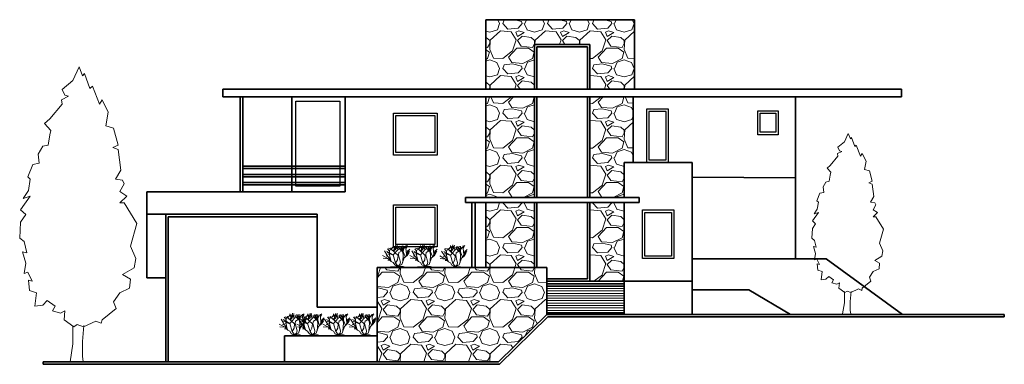
# Model space of a CAD drawing. Units: inches. Extents: x -92 to 721, y 126 to 411.
import ezdxf

# ---------------------------------------------------------------- set-up
doc = ezdxf.new("R2010")
doc.units = ezdxf.units.IN
doc.header["$MEASUREMENT"] = 0
for name, color, linetype, lineweight in [('A-ELEV', 7, 'Continuous', 35), ('A-FLOR-STRS', 3, 'Continuous', 18), ('A-GLAZ', 4, 'Continuous', 25), ('A-WALL-PATT', 8, 'Continuous', 13), ('L-PLNT', 3, 'Continuous', 13)]:
    doc.layers.add(name, color=color, linetype=linetype, lineweight=lineweight)

# ---------------------------------------------------------------- blocks, each defined once
blk = doc.blocks.new('*U2')
blk.add_lwpolyline([(-2.754, 191.699), (-6.78, 182.851), (-13.682, 176.953), (-11.956, 173.266), (-9.656, 172.529), (-14.257, 170.317), (-13.682, 167.368), (-21.733, 157.783), (-25.184, 154.834), (-21.158, 150.41), (-21.733, 147.461), (-22.884, 140.825), (-26.334, 140.087), (-29.21, 134.926), (-28.635, 129.028), (-32.661, 128.291), (-36.111, 120.18), (-34.386, 118.706), (-35.536, 111.333), (-38.987, 106.171), (-34.386, 107.646), (-40.712, 98.798), (-37.261, 95.849), (-40.712, 90.688), (-41.287, 80.366), (-38.412, 78.154), (-36.686, 70.781), (-39.562, 71.518), (-37.261, 64.145), (-38.412, 57.509), (-36.111, 58.247), (-33.236, 52.348), (-35.536, 53.086), (-34.961, 46.45), (-30.36, 44.975), (-31.51, 36.128), (-26.334, 36.865), (-23.459, 39.814), (-18.283, 36.128), (-20.008, 33.178), (-14.832, 31.704), (-11.956, 33.178), (-12.531, 27.28), (-6.205, 22.856), (-3.905, 24.331), (0.121, 22.856), (8.173, 26.543), (11.624, 25.068), (12.199, 27.28), (21.4, 34.653), (19.675, 39.077), (23.701, 44.975), (30.027, 47.924), (30.602, 53.823), (25.426, 56.772), (32.903, 61.196), (34.053, 67.094), (30.602, 75.205), (34.628, 89.951), (26.576, 103.222), (23.701, 103.222), (28.302, 107.646), (23.701, 110.595), (26.576, 115.756), (25.426, 117.968), (20.825, 118.706), (24.276, 124.604), (22.551, 137.876), (19.1, 139.35), (22.551, 140.825), (19.675, 151.884), (14.499, 153.359), (16.224, 162.207), (12.199, 170.317), (10.473, 167.368), (5.872, 179.165), (4.147, 177.69), (0.696, 187.275), (-0.454, 185.8)], close=True)
for points in [[(-6.813, 23.669), (-6.813, 11.669), (-8.627, 0)], [(0.387, 23.669), (-0.576, 13.271), (-0.576, 3.686), (0, 0)]]:
    blk.add_lwpolyline(points)
blk = doc.blocks.new('*U3')
for p, q in [((-14.88, 18.24), (-12.96, 20.64)), ((-12.471, 19.775), (-12.898, 22.044)), ((-11.677, 19.071), (-12.471, 19.775)), ((-11.28, 19.619), (-12.104, 21.184)), ((-11.921, 18.836), (-10.64, 20.401)), ((-11.433, 18.289), (-10.457, 22.749)), ((-10.579, 18.054), (-9.846, 19.697)), ((-8.16, 17.76), (-10.56, 21.6)), ((-9.48, 19.775), (-8.992, 22.592)), ((-7.2, 19.68), (-8.64, 20.16)), ((-7.2, 19.68), (-6.24, 21.12)), ((-5.086, 17.741), (-5.513, 21.34)), ((-5.28, 19.2), (-3.84, 21.6)), ((-3.84, 16.8), (-0.96, 20.64)), ((-3.377, 18.602), (-2.888, 21.575)), ((-2.88, 15.84), (-2.4, 20.16)), ((-0.508, 21.888), (-0.081, 20.558)), ((-0.203, 19.149), (0.102, 21.34)), ((-0.142, 19.384), (0.59, 20.401)), ((-0.02, 20.01), (0.896, 21.105)), ((0.041, 20.714), (1.384, 22.044)), ((0.102, 21.34), (0.835, 21.888)), ((-17.76, 8.64), (-23.663, 11.961)), ((-18.24, 11.04), (-21.755, 16.655)), ((-18.24, 11.04), (-20.16, 11.52)), ((-12.96, 12.48), (-19.68, 16.32)), ((-13.92, 12.48), (-19.2, 14.88)), ((-16.8, 16.32), (-18.72, 18.72)), ((-15.84, 8.16), (-18.24, 11.04)), ((-14.88, 18.24), (-17.76, 19.2)), ((-16.8, 12.48), (-17.76, 12.96)), ((-16.8, 16.32), (-15.36, 19.68)), ((-16.8, 12.48), (-16.8, 16.32)), ((-15.84, 8.16), (-16.8, 12.48)), ((-8.16, 12), (-14.88, 18.24)), ((-12.96, 12.48), (-13.92, 12.48)), ((-13.325, 16.724), (-11.433, 18.289)), ((-12.96, 12.48), (-8.16, 17.76)), ((-10.56, 4.32), (-12.96, 12.48)), ((-12.043, 15.628), (-11.921, 18.836)), ((-11.982, 16.802), (-10.579, 18.054)), ((-8.64, 7.68), (-8.16, 12)), ((-8.16, 17.76), (-5.28, 19.2)), ((-7.68, 12.48), (-7.2, 14.88)), ((-6.72, 8.64), (-7.68, 12.48)), ((-4.8, 16.32), (-7.2, 19.68)), ((-7.2, 14.88), (-3.84, 16.8)), ((-3.377, 15.315), (-5.086, 17.819)), ((-2.88, 12.96), (-4.32, 19.68)), ((-2.766, 16.802), (-3.377, 18.602)), ((-3.36, 5.28), (-2.88, 12.96)), ((-0.96, 10.56), (-2.88, 15.84)), ((-1.92, 9.6), (0.96, 12)), ((-0.48, 10.8), (0.346, 13.203)), ((0.346, 13.203), (-0.203, 19.149)), ((0.346, 13.203), (1.323, 16.254)), ((0.96, 12), (1.44, 15.36)), ((0.96, 12), (2.88, 14.88)), ((1.323, 16.254), (3.642, 18.289)), ((1.44, 15.36), (2.88, 17.28)), ((1.92, 13.44), (2.4, 15.36)), ((2.4, 15.36), (3.36, 16.32)), ((-17.76, 8.64), (-23.128, 9.222)), ((-16.32, 7.2), (-18.24, 7.2)), ((-14.88, 5.76), (-17.76, 8.64)), ((-15.84, 0.48), (-17.76, 0)), ((-14.88, 5.76), (-15.84, 8.16)), ((-13.44, 0.48), (-15.84, 0.48)), ((-12.96, 4.8), (-14.88, 5.76)), ((-9.6, 0.96), (-13.44, 0.48)), ((-11.52, 2.4), (-12.96, 4.8)), ((-9.6, 0.96), (-12.96, 0)), ((-8.64, 0.96), (-11.52, 2.4)), ((-10.56, 4.32), (-8.64, 7.68)), ((-8.64, 1.92), (-10.56, 4.32)), ((-9.6, 0.96), (-7.68, 0.96)), ((-8.64, 0.96), (-4.32, 2.88)), ((-8.64, 0.96), (-6.24, 2.88)), ((-8.64, 0.96), (-8.64, 1.92)), ((-8.64, 0.96), (-2.88, 0.96)), ((-7.68, 0.96), (-6.24, 0.48)), ((-5.76, 5.28), (-6.72, 8.64)), ((-6.24, 2.88), (-5.76, 5.28)), ((-6.24, 0.48), (-3.36, 0)), ((-4.32, 2.88), (-1.92, 9.6)), ((-2.88, 0.96), (0, 0))]:
    blk.add_line(p, q)

msp = doc.modelspace()

# ---------------------------------------------------------------- hatches: boundary and pattern name
at = {"layer": 'A-WALL-PATT'}
h = msp.add_hatch(dxfattribs=at)
h.set_pattern_fill('GRAVEL', color=256, scale=37)
h.paths.add_polyline_path([(343.25, 205.86), (203.17, 205.86), (203.17, 127.76), (303.34, 127.76), (343.25, 166.98)])
h.paths.add_polyline_path([(333.11, 259.5), (293.07, 259.5), (293.07, 205.86), (333.11, 205.86)])
h.paths.add_polyline_path([(333.11, 346.84), (293.07, 346.84), (293.07, 263.5), (333.11, 263.5)])
h.paths.add_polyline_path([(333.11, 388.04), (333.11, 390.04), (335.11, 390.04), (376.85, 390.04), (378.85, 390.04), (378.85, 388.04), (378.85, 353.03), (415.66, 353.03), (415.66, 410.52), (293.07, 410.52), (293.07, 353.03), (333.11, 353.03)])
h.paths.add_polyline_path([(414.62, 346.84), (378.85, 346.84), (378.85, 263.5), (407.16, 263.5), (407.16, 280.35), (407.16, 292.58), (414.62, 292.58)])
h.paths.add_polyline_path([(407.16, 259.5), (378.85, 259.5), (378.85, 194.36), (407.16, 194.36)])

# ---------------------------------------------------------------- linework, layer by layer
at = {"layer": 'A-ELEV'}
for p, q in [((293.07, 353.03), (293.07, 410.52)), ((293.07, 410.52), (415.66, 410.52)), ((415.66, 410.52), (415.66, 353.03)), ((333.11, 388.04), (333.11, 390.04)), ((333.11, 390.04), (335.11, 390.04)), ((333.11, 353.03), (333.11, 388.04)), ((335.11, 390.04), (376.85, 390.04)), ((335.11, 353.03), (335.11, 388.04)), ((335.11, 388.04), (376.85, 388.04)), ((376.85, 390.04), (378.85, 390.04)), ((376.85, 388.04), (376.85, 353.03)), ((378.85, 390.04), (378.85, 388.04)), ((378.85, 388.04), (378.85, 353.03)), ((76.04, 349.84), (76.04, 353.03)), ((76.04, 353.03), (221.72, 353.03)), ((76.04, 346.84), (76.04, 349.84)), ((221.72, 353.03), (456.3, 353.03)), ((456.3, 353.03), (636.01, 353.03)), ((636.01, 346.84), (636.01, 353.03)), ((92.35, 346.84), (76.04, 346.84)), ((90.35, 268.23), (90.35, 346.84)), ((92.35, 268.23), (92.35, 346.84)), ((92.35, 346.84), (222.07, 346.84)), ((132.94, 346.84), (132.94, 268.23)), ((176.92, 268.23), (176.92, 346.84)), ((222.07, 346.84), (461.09, 346.84)), ((293.07, 263.5), (293.07, 346.84)), ((333.11, 346.84), (333.11, 263.5)), ((335.11, 346.84), (335.11, 263.5)), ((376.85, 346.84), (376.85, 263.5)), ((378.85, 346.84), (378.85, 263.5)), ((414.62, 346.84), (414.62, 292.58)), ((461.09, 346.84), (636.01, 346.84)), ((548.6, 346.84), (548.6, 212.92)), ((407.16, 292.58), (463.17, 292.58)), ((407.16, 292.58), (407.16, 280.35)), ((463.17, 292.58), (463.17, 280.35)), ((92.35, 289.45), (176.92, 289.45)), ((92.35, 287.45), (176.92, 287.45)), ((92.35, 282.7), (176.92, 282.7)), ((92.35, 280.7), (176.92, 280.7)), ((407.16, 263.5), (407.16, 280.35)), ((463.17, 280.35), (463.17, 194.36)), ((463.17, 280.35), (548.6, 279.88)), ((13.32, 249.76), (13.32, 268.23)), ((13.32, 268.23), (90.35, 268.23)), ((90.35, 268.23), (176.92, 268.23)), ((92.35, 276.06), (176.92, 276.06)), ((92.35, 274.06), (176.92, 274.06)), ((293.07, 263.5), (276.26, 263.5)), ((276.26, 263.5), (276.26, 259.5)), ((293.07, 263.5), (407.16, 263.5)), ((407.16, 263.5), (419.4, 263.5)), ((419.4, 263.5), (419.4, 259.5)), ((276.26, 259.5), (293.07, 259.5)), ((281.29, 259.5), (281.29, 205.86)), ((284.29, 259.5), (284.29, 205.86)), ((293.07, 205.86), (293.07, 259.5)), ((293.07, 259.5), (407.16, 259.5)), ((333.11, 259.5), (333.11, 205.86)), ((335.11, 259.5), (335.11, 205.86)), ((376.85, 259.5), (376.85, 196.36)), ((378.85, 259.5), (378.85, 194.36)), ((407.16, 194.36), (407.16, 259.5)), ((419.4, 259.5), (407.16, 259.5)), ((13.32, 197.1), (13.32, 249.76)), ((13.32, 249.76), (28.77, 249.76)), ((28.77, 247.76), (28.77, 249.76)), ((28.77, 249.76), (29.94, 249.76)), ((28.77, 127.76), (28.77, 247.76)), ((29.94, 249.76), (30.77, 249.76)), ((30.77, 249.76), (153.85, 249.76)), ((30.77, 127.76), (30.77, 247.76)), ((30.77, 247.76), (153.85, 247.76)), ((153.85, 247.76), (153.85, 249.76)), ((153.85, 247.76), (153.85, 184.21)), ((463.17, 212.92), (573.83, 212.92)), ((573.83, 212.92), (636.98, 166.98)), ((343.25, 205.86), (203.17, 205.86)), ((203.17, 205.86), (203.17, 127.76)), ((343.25, 166.98), (343.25, 205.86)), ((28.77, 197.1), (13.32, 197.1)), ((376.85, 196.36), (343.25, 196.36)), ((407.16, 194.36), (343.25, 194.36)), ((407.16, 192.36), (343.25, 192.36)), ((407.16, 190.36), (343.25, 190.36)), ((463.17, 194.36), (407.16, 194.36)), ((407.16, 194.36), (407.16, 166.98)), ((463.17, 194.36), (463.17, 166.98)), ((463.17, 187.43), (509.98, 187.43)), ((509.98, 187.43), (544.34, 166.98)), ((153.85, 184.21), (153.85, 172.87)), ((153.85, 172.87), (203.17, 172.87)), ((407.16, 168.36), (343.25, 168.36)), ((720.87, 164.98), (720.87, 166.98)), ((203.17, 149.21), (126.87, 149.21)), ((126.87, 149.21), (126.87, 127.76)), ((-72.48, 125.76), (-72.48, 127.76))]:
    msp.add_line(p, q, dxfattribs=at)
for points in [[(-72.48, 127.76), (67.29, 127.76), (303.34, 127.76), (343.25, 166.98), (720.87, 166.98)], [(-72.48, 125.76), (67.29, 125.76), (304.16, 125.76), (344.07, 164.98), (720.87, 164.98)]]:
    msp.add_lwpolyline(points, dxfattribs=at)
at = {"layer": 'A-FLOR-STRS'}
for p, q in [((407.16, 188.36), (343.25, 188.36)), ((407.16, 186.36), (343.25, 186.36)), ((407.16, 184.36), (343.25, 184.36)), ((407.16, 182.36), (343.25, 182.36)), ((407.16, 180.36), (343.25, 180.36)), ((407.16, 178.36), (343.25, 178.36)), ((407.16, 176.36), (343.25, 176.36)), ((407.16, 174.36), (343.25, 174.36)), ((407.16, 172.36), (343.25, 172.36)), ((407.16, 170.36), (343.25, 170.36))]:
    msp.add_line(p, q, dxfattribs=at)
at = {"layer": 'A-GLAZ'}
for points in [[(136.14, 343.3), (172.55, 343.3), (172.55, 272.86), (136.14, 272.86)], [(216.82, 333.24), (252.92, 333.24), (252.92, 298.65), (216.82, 298.65)], [(425.6, 292.58), (443.68, 292.58), (443.68, 336.57), (425.6, 336.57)], [(427.6, 294.58), (441.68, 294.58), (441.68, 334.57), (427.6, 334.57)], [(517.5, 335.31), (534.32, 335.31), (534.32, 315.49), (517.5, 315.49)], [(519.5, 333.31), (532.32, 333.31), (532.32, 317.49), (519.5, 317.49)], [(218.82, 331.24), (250.92, 331.24), (250.92, 300.65), (218.82, 300.65)], [(216.82, 257.65), (252.92, 257.65), (252.92, 222.78), (216.82, 222.78)], [(218.82, 255.65), (250.92, 255.65), (250.92, 224.78), (218.82, 224.78)], [(422.29, 253.27), (448.11, 253.27), (448.11, 213.24), (422.29, 213.24)], [(424.29, 251.27), (446.11, 251.27), (446.11, 215.24), (424.29, 215.24)]]:
    msp.add_lwpolyline(points, close=True, dxfattribs=at)

# ---------------------------------------------------------------- block references
at = {"layer": 'L-PLNT'}
for name, p, xscale, yscale, zscale in [('*U2', (-39.22, 127.76), 1.27197040701415, 1.27197040701415, 1.27197040701415), ('*U2', (594.17, 167.39), 0.7781149511396727, 0.7781149511396727, 0.7781149511396727), ('*U3', (227.25, 205.86), 0.8251920061282577, 0.8251920061282577, 0.8251920061282577), ('*U3', (249.74, 205.86), 0.8251920061282577, 0.8251920061282577, 0.8251920061282577), ('*U3', (274.44, 205.63), 0.8251920061282577, 0.8251920061282577, 0.8251920061282577), ('*U3', (141.93, 149.21), 0.8251920061282577, 0.8251920061282577, 0.8251920061282577), ('*U3', (156.59, 149.21), 0.8251920061282577, 0.8251920061282577, 0.8251920061282577), ('*U3', (177.85, 149.21), 0.8251920061282577, 0.8251920061282577, 0.8251920061282577), ('*U3', (199.29, 149.21), 0.8251920061282577, 0.8251920061282577, 0.8251920061282577)]:
    msp.add_blockref(name, p, dxfattribs=dict(at, xscale=xscale, yscale=yscale, zscale=zscale))

doc.saveas('drawing.dxf')
